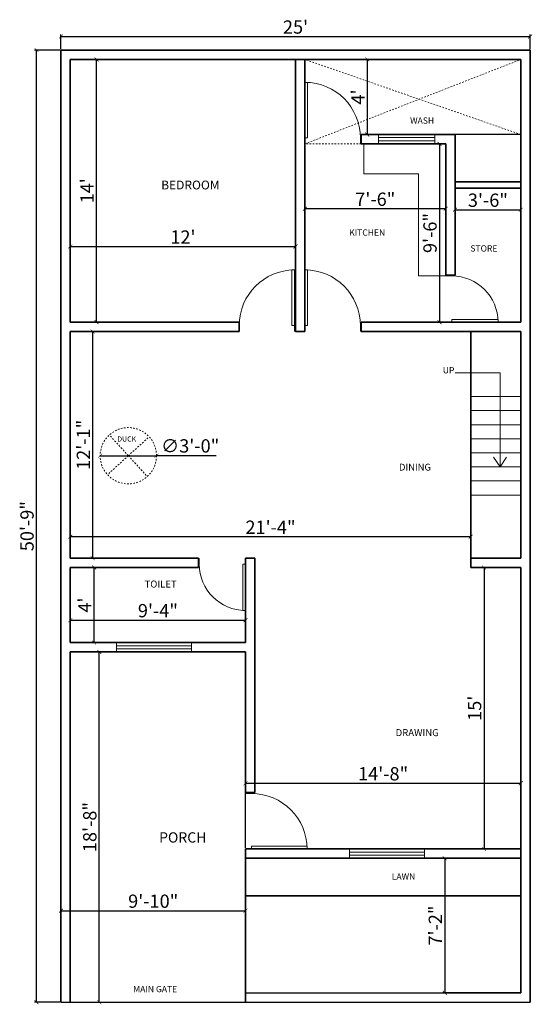
# Model space of a CAD drawing. Units: inches. Extents: x 3799 to 20199, y 1682 to 8087.
# Tile 22 of 30: x 12191 to 12519, y 6979 to 7609. Entities that reach past the tile are written whole.
import ezdxf

# ---------------------------------------------------------------- set-up
doc = ezdxf.new("R2010")
doc.units = ezdxf.units.IN
doc.linetypes.add('JIS_02_1.0', pattern=[2, 1, -1])
for name, color, linetype, lineweight in [('A-ANNO-DIMS', 2, 'Continuous', 18), ('A-ANNO-SYMB', 3, 'Continuous', 18), ('A-AREA-IDEN', 7, 'Continuous', 18), ('A-DOOR', 3, 'Continuous', 18), ('A-FLOR-CASE', 32, 'Continuous', 18), ('A-FLOR-SHFT-HIDN', 8, 'JIS_02_1.0', 13), ('A-FLOR-STRS', 41, 'Continuous', 18), ('A-GLAZ', 152, 'Continuous', 18), ('A-WALL', 7, 'Continuous', 35), ('A-WALL-OVHD', 7, 'JIS_02_1.0', 18), ('C-PROP', 7, 'Continuous', 25)]:
    doc.layers.add(name, color=color, linetype=linetype, lineweight=lineweight)
doc.styles.get("Standard").update_dxf_attribs({"font": 'arial.ttf'})
doc.dimstyles.new('ISO-25', dxfattribs={"dimtxt": 8.5, "dimasz": 2.5, "dimexe": 1.25, "dimexo": 0.625, "dimtad": 1, "dimdec": 0, "dimlunit": 3, "dimtxsty": 'Standard', "dimblk": 'ARCHTICK', "dimcen": 2.5, "dimadec": 0, "dimazin": 0, "dimtfac": 1, "dimtdec": 0, "dimtmove": 0, "dimatfit": 3, "dimfxl": 1, "dimarcsym": 0})

# ---------------------------------------------------------------- blocks, each defined once
blk = doc.blocks.new('_ArchTick')
at = {"color": 0, "linetype": 'ByBlock', "const_width": 0.15}
blk.add_lwpolyline([(-0.5, -0.5), (0.5, 0.5)], dxfattribs=at)
blk = doc.blocks.new('*D177')
at = {"layer": 'A-ANNO-DIMS', "color": 0, "lineweight": -2, "transparency": 16777216}
for p, q in [((12217.15, 7590.06), (12217.15, 7599.38)), ((12217.15, 7598.13), (12517.15, 7598.13)), ((12517.15, 7590.06), (12517.15, 7599.38))]:
    blk.add_line(p, q, dxfattribs=at)
at = {"layer": 'Defpoints', "color": 0, "transparency": 16777216}
for p in [(12517.15, 7598.13), (12217.15, 7589.44), (12517.15, 7589.44)]:
    blk.add_point(p, dxfattribs=at)
at = {"layer": 'A-ANNO-DIMS', "color": 0, "lineweight": -2, "transparency": 16777216, "xscale": 2.5, "yscale": 2.5, "zscale": 2.5, "rotation": 180}
blk.add_blockref('_ArchTick', (12217.15, 7598.13), dxfattribs=at)
at = {"layer": 'A-ANNO-DIMS', "color": 0, "lineweight": -2, "transparency": 16777216, "xscale": 2.5, "yscale": 2.5, "zscale": 2.5}
blk.add_blockref('_ArchTick', (12517.15, 7598.13), dxfattribs=at)
at = {"layer": 'A-ANNO-DIMS', "color": 0, "transparency": 16777216, "insert": (12367.15, 7603.1), "char_height": 8.5, "attachment_point": 5}
blk.add_mtext("25'", dxfattribs=at)
blk = doc.blocks.new('*D178')
at = {"layer": 'A-ANNO-DIMS', "color": 0, "lineweight": -2, "transparency": 16777216}
for p, q in [((12216.53, 7589.44), (12200.29, 7589.44)), ((12201.54, 6980.44), (12201.54, 7589.44)), ((12216.53, 6980.44), (12200.29, 6980.44))]:
    blk.add_line(p, q, dxfattribs=at)
at = {"layer": 'Defpoints', "color": 0, "transparency": 16777216}
for p in [(12201.54, 7589.44), (12217.15, 7589.44), (12217.15, 6980.44)]:
    blk.add_point(p, dxfattribs=at)
at = {"layer": 'A-ANNO-DIMS', "color": 0, "lineweight": -2, "transparency": 16777216, "xscale": 2.5, "yscale": 2.5, "zscale": 2.5}
for p, rotation in [((12201.54, 7589.44), 90), ((12201.54, 6980.44), 270)]:
    blk.add_blockref('_ArchTick', p, dxfattribs=dict(at, rotation=rotation))
at = {"layer": 'A-ANNO-DIMS', "color": 0, "transparency": 16777216, "insert": (12196.57, 7284.94), "char_height": 8.5, "attachment_point": 5, "rotation": 90}
blk.add_mtext('50\'-9"', dxfattribs=at)
blk = doc.blocks.new('*U49')
for p, q in [((0, 0), (0, -100)), ((900, 0), (900, -100))]:
    blk.add_line(p, q)
blk.add_lwpolyline([(0, 0), (0, 900), (43.75, 900), (43.75, 0)], close=True)
blk.add_arc((0, 0), 900, 0, 90)
blk = doc.blocks.new('*U171')
for p, q in [((-750, 0), (-750, 100)), ((0, 0), (0, 100))]:
    blk.add_line(p, q)
blk.add_lwpolyline([(0, 0), (0, -750), (-43.75, -750), (-43.75, 0)], close=True)
blk.add_arc((0, 0), 750, 180, 270)
blk = doc.blocks.new('*U179')
for p, q in [((0, 0), (0, -100)), ((-900, 0), (-900, -100))]:
    blk.add_line(p, q)
blk.add_lwpolyline([(0, 0), (0, 900), (-43.75, 900), (-43.75, 0)], close=True)
blk.add_arc((0, 0), 900, 90, 180)
blk = doc.blocks.new('*U148')
for p, q in [((-750, 0), (-750, -100)), ((0, 0), (0, -100))]:
    blk.add_line(p, q)
blk.add_lwpolyline([(0, 0), (0, 750), (-43.75, 750), (-43.75, 0)], close=True)
blk.add_arc((0, 0), 750, 90, 180)
blk = doc.blocks.new('*D181')
at = {"layer": 'A-ANNO-DIMS', "color": 0, "lineweight": -2, "transparency": 16777216}
for p, q in [((12223.78, 7583.44), (12241.14, 7583.44)), ((12239.89, 7415.44), (12239.89, 7583.44)), ((12223.78, 7415.44), (12241.14, 7415.44))]:
    blk.add_line(p, q, dxfattribs=at)
at = {"layer": 'Defpoints', "color": 0, "transparency": 16777216}
for p in [(12223.15, 7583.44), (12239.89, 7583.44), (12223.15, 7415.44)]:
    blk.add_point(p, dxfattribs=at)
at = {"layer": 'A-ANNO-DIMS', "color": 0, "lineweight": -2, "transparency": 16777216, "xscale": 2.5, "yscale": 2.5, "zscale": 2.5}
for p, rotation in [((12239.89, 7583.44), 90), ((12239.89, 7415.44), 270)]:
    blk.add_blockref('_ArchTick', p, dxfattribs=dict(at, rotation=rotation))
at = {"layer": 'A-ANNO-DIMS', "color": 0, "transparency": 16777216, "insert": (12235, 7499.44), "char_height": 8.5, "attachment_point": 5, "rotation": 90}
blk.add_mtext("14'", dxfattribs=at)
blk = doc.blocks.new('*D182')
at = {"layer": 'A-ANNO-DIMS', "color": 0, "lineweight": -2, "transparency": 16777216}
for p, q in [((12223.15, 7582.81), (12223.15, 7462.61)), ((12367.15, 7582.81), (12367.15, 7462.61)), ((12223.15, 7463.86), (12367.15, 7463.86))]:
    blk.add_line(p, q, dxfattribs=at)
at = {"layer": 'Defpoints', "color": 0, "transparency": 16777216}
for p in [(12223.15, 7583.44), (12367.15, 7583.44), (12367.15, 7463.86)]:
    blk.add_point(p, dxfattribs=at)
at = {"layer": 'A-ANNO-DIMS', "color": 0, "lineweight": -2, "transparency": 16777216, "xscale": 2.5, "yscale": 2.5, "zscale": 2.5, "rotation": 180}
blk.add_blockref('_ArchTick', (12223.15, 7463.86), dxfattribs=at)
at = {"layer": 'A-ANNO-DIMS', "color": 0, "lineweight": -2, "transparency": 16777216, "xscale": 2.5, "yscale": 2.5, "zscale": 2.5}
blk.add_blockref('_ArchTick', (12367.15, 7463.86), dxfattribs=at)
at = {"layer": 'A-ANNO-DIMS', "color": 0, "transparency": 16777216, "insert": (12295.15, 7468.75), "char_height": 8.5, "attachment_point": 5}
blk.add_mtext("12'", dxfattribs=at)
blk = doc.blocks.new('*D183')
at = {"layer": 'A-ANNO-DIMS', "color": 0, "lineweight": -2, "transparency": 16777216}
for p, q in [((12510.53, 7583.44), (12411.75, 7583.44)), ((12413, 7583.44), (12413, 7535.44)), ((12510.53, 7535.44), (12411.75, 7535.44))]:
    blk.add_line(p, q, dxfattribs=at)
at = {"layer": 'Defpoints', "color": 0, "transparency": 16777216}
for p in [(12511.15, 7583.44), (12413, 7535.44), (12511.15, 7535.44)]:
    blk.add_point(p, dxfattribs=at)
at = {"layer": 'A-ANNO-DIMS', "color": 0, "lineweight": -2, "transparency": 16777216, "xscale": 2.5, "yscale": 2.5, "zscale": 2.5}
for p, rotation in [((12413, 7583.44), 90), ((12413, 7535.44), 270)]:
    blk.add_blockref('_ArchTick', p, dxfattribs=dict(at, rotation=rotation))
at = {"layer": 'A-ANNO-DIMS', "color": 0, "transparency": 16777216, "insert": (12408.12, 7559.44), "char_height": 8.5, "attachment_point": 5, "rotation": 90}
blk.add_mtext("4'", dxfattribs=at)
blk = doc.blocks.new('*D184')
at = {"layer": 'A-ANNO-DIMS', "color": 0, "lineweight": -2, "transparency": 16777216}
for p, q in [((12373.15, 7446.06), (12373.15, 7489.23)), ((12463.15, 7446.06), (12463.15, 7489.23)), ((12463.15, 7487.98), (12373.15, 7487.98))]:
    blk.add_line(p, q, dxfattribs=at)
at = {"layer": 'Defpoints', "color": 0, "transparency": 16777216}
for p in [(12373.15, 7487.98), (12373.15, 7445.44), (12463.15, 7445.44)]:
    blk.add_point(p, dxfattribs=at)
at = {"layer": 'A-ANNO-DIMS', "color": 0, "lineweight": -2, "transparency": 16777216, "xscale": 2.5, "yscale": 2.5, "zscale": 2.5, "rotation": 180}
blk.add_blockref('_ArchTick', (12373.15, 7487.98), dxfattribs=at)
at = {"layer": 'A-ANNO-DIMS', "color": 0, "lineweight": -2, "transparency": 16777216, "xscale": 2.5, "yscale": 2.5, "zscale": 2.5}
blk.add_blockref('_ArchTick', (12463.15, 7487.98), dxfattribs=at)
at = {"layer": 'A-ANNO-DIMS', "color": 0, "transparency": 16777216, "insert": (12418.15, 7492.95), "char_height": 8.5, "attachment_point": 5}
blk.add_mtext('7\'-6"', dxfattribs=at)
blk = doc.blocks.new('*D185')
at = {"layer": 'A-ANNO-DIMS', "color": 0, "lineweight": -2, "transparency": 16777216}
for p, q in [((12462.53, 7529.44), (12457.95, 7529.44)), ((12459.2, 7529.44), (12459.2, 7415.44)), ((12462.53, 7415.44), (12457.95, 7415.44))]:
    blk.add_line(p, q, dxfattribs=at)
at = {"layer": 'Defpoints', "color": 0, "transparency": 16777216}
for p in [(12463.15, 7529.44), (12459.2, 7415.44), (12463.15, 7415.44)]:
    blk.add_point(p, dxfattribs=at)
at = {"layer": 'A-ANNO-DIMS', "color": 0, "lineweight": -2, "transparency": 16777216, "xscale": 2.5, "yscale": 2.5, "zscale": 2.5}
for p, rotation in [((12459.2, 7529.44), 90), ((12459.2, 7415.44), 270)]:
    blk.add_blockref('_ArchTick', p, dxfattribs=dict(at, rotation=rotation))
at = {"layer": 'A-ANNO-DIMS', "color": 0, "transparency": 16777216, "insert": (12454.24, 7472.44), "char_height": 8.5, "attachment_point": 5, "rotation": 90}
blk.add_mtext('9\'-6"', dxfattribs=at)
blk = doc.blocks.new('*D186')
at = {"layer": 'A-ANNO-DIMS', "color": 0, "lineweight": -2, "transparency": 16777216}
for p, q in [((12469.15, 7500.59), (12469.15, 7486.11)), ((12511.15, 7500.59), (12511.15, 7486.11)), ((12469.15, 7487.36), (12511.15, 7487.36))]:
    blk.add_line(p, q, dxfattribs=at)
at = {"layer": 'Defpoints', "color": 0, "transparency": 16777216}
for p in [(12469.15, 7501.21), (12511.15, 7501.21), (12511.15, 7487.36)]:
    blk.add_point(p, dxfattribs=at)
at = {"layer": 'A-ANNO-DIMS', "color": 0, "lineweight": -2, "transparency": 16777216, "xscale": 2.5, "yscale": 2.5, "zscale": 2.5, "rotation": 180}
blk.add_blockref('_ArchTick', (12469.15, 7487.36), dxfattribs=at)
at = {"layer": 'A-ANNO-DIMS', "color": 0, "lineweight": -2, "transparency": 16777216, "xscale": 2.5, "yscale": 2.5, "zscale": 2.5}
blk.add_blockref('_ArchTick', (12511.15, 7487.36), dxfattribs=at)
at = {"layer": 'A-ANNO-DIMS', "color": 0, "transparency": 16777216, "insert": (12490.15, 7492.33), "char_height": 8.5, "attachment_point": 5}
blk.add_mtext('3\'-6"', dxfattribs=at)
blk = doc.blocks.new('*D187')
at = {"layer": 'A-ANNO-DIMS', "color": 0, "lineweight": -2, "transparency": 16777216}
for p, q in [((12223.78, 7409.44), (12238.72, 7409.44)), ((12237.47, 7264.44), (12237.47, 7409.44)), ((12223.78, 7264.44), (12238.72, 7264.44))]:
    blk.add_line(p, q, dxfattribs=at)
at = {"layer": 'Defpoints', "color": 0, "transparency": 16777216}
for p in [(12223.15, 7409.44), (12237.47, 7409.44), (12223.15, 7264.44)]:
    blk.add_point(p, dxfattribs=at)
at = {"layer": 'A-ANNO-DIMS', "color": 0, "lineweight": -2, "transparency": 16777216, "xscale": 2.5, "yscale": 2.5, "zscale": 2.5}
for p, rotation in [((12237.47, 7409.44), 90), ((12237.47, 7264.44), 270)]:
    blk.add_blockref('_ArchTick', p, dxfattribs=dict(at, rotation=rotation))
at = {"layer": 'A-ANNO-DIMS', "color": 0, "transparency": 16777216, "insert": (12232.58, 7336.94), "char_height": 8.5, "attachment_point": 5, "rotation": 90}
blk.add_mtext('12\'-1"', dxfattribs=at)
blk = doc.blocks.new('*D188')
at = {"layer": 'A-ANNO-DIMS', "color": 0, "lineweight": -2, "transparency": 16777216}
for p, q in [((12223.15, 7265.06), (12223.15, 7279.48)), ((12223.15, 7278.23), (12479.15, 7278.23)), ((12479.15, 7265.06), (12479.15, 7279.48))]:
    blk.add_line(p, q, dxfattribs=at)
at = {"layer": 'Defpoints', "color": 0, "transparency": 16777216}
for p in [(12479.15, 7278.23), (12223.15, 7264.44), (12479.15, 7264.44)]:
    blk.add_point(p, dxfattribs=at)
at = {"layer": 'A-ANNO-DIMS', "color": 0, "lineweight": -2, "transparency": 16777216, "xscale": 2.5, "yscale": 2.5, "zscale": 2.5, "rotation": 180}
blk.add_blockref('_ArchTick', (12223.15, 7278.23), dxfattribs=at)
at = {"layer": 'A-ANNO-DIMS', "color": 0, "lineweight": -2, "transparency": 16777216, "xscale": 2.5, "yscale": 2.5, "zscale": 2.5}
blk.add_blockref('_ArchTick', (12479.15, 7278.23), dxfattribs=at)
at = {"layer": 'A-ANNO-DIMS', "color": 0, "transparency": 16777216, "insert": (12351.15, 7283.12), "char_height": 8.5, "attachment_point": 5}
blk.add_mtext('21\'-4"', dxfattribs=at)
blk = doc.blocks.new('*D189')
at = {"layer": 'A-ANNO-DIMS', "color": 0, "lineweight": -2, "transparency": 16777216}
for p, q in [((12223.78, 7258.44), (12239.64, 7258.44)), ((12238.39, 7210.44), (12238.39, 7258.44)), ((12223.78, 7210.44), (12239.64, 7210.44))]:
    blk.add_line(p, q, dxfattribs=at)
at = {"layer": 'Defpoints', "color": 0, "transparency": 16777216}
for p in [(12223.15, 7258.44), (12238.39, 7258.44), (12223.15, 7210.44)]:
    blk.add_point(p, dxfattribs=at)
at = {"layer": 'A-ANNO-DIMS', "color": 0, "lineweight": -2, "transparency": 16777216, "xscale": 2.5, "yscale": 2.5, "zscale": 2.5}
for p, rotation in [((12238.39, 7258.44), 90), ((12238.39, 7210.44), 270)]:
    blk.add_blockref('_ArchTick', p, dxfattribs=dict(at, rotation=rotation))
at = {"layer": 'A-ANNO-DIMS', "color": 0, "transparency": 16777216, "insert": (12233.52, 7234.44), "char_height": 8.5, "attachment_point": 5, "rotation": 90}
blk.add_mtext("4'", dxfattribs=at)
blk = doc.blocks.new('*D190')
at = {"layer": 'A-ANNO-DIMS', "color": 0, "lineweight": -2, "transparency": 16777216}
for p, q in [((12223.15, 7211.06), (12223.15, 7226.05)), ((12223.15, 7224.8), (12335.15, 7224.8)), ((12335.15, 7211.06), (12335.15, 7226.05))]:
    blk.add_line(p, q, dxfattribs=at)
at = {"layer": 'Defpoints', "color": 0, "transparency": 16777216}
for p in [(12335.15, 7224.8), (12223.15, 7210.44), (12335.15, 7210.44)]:
    blk.add_point(p, dxfattribs=at)
at = {"layer": 'A-ANNO-DIMS', "color": 0, "lineweight": -2, "transparency": 16777216, "xscale": 2.5, "yscale": 2.5, "zscale": 2.5, "rotation": 180}
blk.add_blockref('_ArchTick', (12223.15, 7224.8), dxfattribs=at)
at = {"layer": 'A-ANNO-DIMS', "color": 0, "lineweight": -2, "transparency": 16777216, "xscale": 2.5, "yscale": 2.5, "zscale": 2.5}
blk.add_blockref('_ArchTick', (12335.15, 7224.8), dxfattribs=at)
at = {"layer": 'A-ANNO-DIMS', "color": 0, "transparency": 16777216, "insert": (12279.15, 7229.76), "char_height": 8.5, "attachment_point": 5}
blk.add_mtext('9\'-4"', dxfattribs=at)
blk = doc.blocks.new('*D191')
at = {"layer": 'A-ANNO-DIMS', "color": 0, "lineweight": -2, "transparency": 16777216}
for p, q in [((12223.78, 7204.44), (12242.92, 7204.44)), ((12241.67, 6980.44), (12241.67, 7204.44)), ((12223.78, 6980.44), (12242.92, 6980.44))]:
    blk.add_line(p, q, dxfattribs=at)
at = {"layer": 'Defpoints', "color": 0, "transparency": 16777216}
for p in [(12223.15, 7204.44), (12241.67, 7204.44), (12223.15, 6980.44)]:
    blk.add_point(p, dxfattribs=at)
at = {"layer": 'A-ANNO-DIMS', "color": 0, "lineweight": -2, "transparency": 16777216, "xscale": 2.5, "yscale": 2.5, "zscale": 2.5}
for p, rotation in [((12241.67, 7204.44), 90), ((12241.67, 6980.44), 270)]:
    blk.add_blockref('_ArchTick', p, dxfattribs=dict(at, rotation=rotation))
at = {"layer": 'A-ANNO-DIMS', "color": 0, "transparency": 16777216, "insert": (12236.71, 7092.44), "char_height": 8.5, "attachment_point": 5, "rotation": 90}
blk.add_mtext('18\'-8"', dxfattribs=at)
blk = doc.blocks.new('*D192')
at = {"layer": 'A-ANNO-DIMS', "color": 0, "lineweight": -2, "transparency": 16777216}
for p, q in [((12217.15, 6981.06), (12217.15, 7040.2)), ((12217.15, 7038.95), (12335.15, 7038.95)), ((12335.15, 6981.06), (12335.15, 7040.2))]:
    blk.add_line(p, q, dxfattribs=at)
at = {"layer": 'Defpoints', "color": 0, "transparency": 16777216}
for p in [(12335.15, 7038.95), (12217.15, 6980.44), (12335.15, 6980.44)]:
    blk.add_point(p, dxfattribs=at)
at = {"layer": 'A-ANNO-DIMS', "color": 0, "lineweight": -2, "transparency": 16777216, "xscale": 2.5, "yscale": 2.5, "zscale": 2.5, "rotation": 180}
blk.add_blockref('_ArchTick', (12217.15, 7038.95), dxfattribs=at)
at = {"layer": 'A-ANNO-DIMS', "color": 0, "lineweight": -2, "transparency": 16777216, "xscale": 2.5, "yscale": 2.5, "zscale": 2.5}
blk.add_blockref('_ArchTick', (12335.15, 7038.95), dxfattribs=at)
at = {"layer": 'A-ANNO-DIMS', "color": 0, "transparency": 16777216, "insert": (12276.15, 7043.92), "char_height": 8.5, "attachment_point": 5}
blk.add_mtext('9\'-10"', dxfattribs=at)
blk = doc.blocks.new('*D193')
at = {"layer": 'A-ANNO-DIMS', "color": 0, "lineweight": -2, "transparency": 16777216}
for p, q in [((12510.53, 7072.44), (12461.27, 7072.44)), ((12462.52, 7072.44), (12462.52, 6986.44)), ((12510.53, 6986.44), (12461.27, 6986.44))]:
    blk.add_line(p, q, dxfattribs=at)
at = {"layer": 'Defpoints', "color": 0, "transparency": 16777216}
for p in [(12511.15, 7072.44), (12462.52, 6986.44), (12511.15, 6986.44)]:
    blk.add_point(p, dxfattribs=at)
at = {"layer": 'A-ANNO-DIMS', "color": 0, "lineweight": -2, "transparency": 16777216, "xscale": 2.5, "yscale": 2.5, "zscale": 2.5}
for p, rotation in [((12462.52, 7072.44), 90), ((12462.52, 6986.44), 270)]:
    blk.add_blockref('_ArchTick', p, dxfattribs=dict(at, rotation=rotation))
at = {"layer": 'A-ANNO-DIMS', "color": 0, "transparency": 16777216, "insert": (12457.63, 7029.44), "char_height": 8.5, "attachment_point": 5, "rotation": 90}
blk.add_mtext('7\'-2"', dxfattribs=at)
blk = doc.blocks.new('*D194')
at = {"layer": 'A-ANNO-DIMS', "color": 0, "lineweight": -2, "transparency": 16777216}
for p, q in [((12510.53, 7258.44), (12486.45, 7258.44)), ((12487.7, 7258.44), (12487.7, 7078.44)), ((12510.53, 7078.44), (12486.45, 7078.44))]:
    blk.add_line(p, q, dxfattribs=at)
at = {"layer": 'Defpoints', "color": 0, "transparency": 16777216}
for p in [(12511.15, 7258.44), (12487.7, 7078.44), (12511.15, 7078.44)]:
    blk.add_point(p, dxfattribs=at)
at = {"layer": 'A-ANNO-DIMS', "color": 0, "lineweight": -2, "transparency": 16777216, "xscale": 2.5, "yscale": 2.5, "zscale": 2.5}
for p, rotation in [((12487.7, 7258.44), 90), ((12487.7, 7078.44), 270)]:
    blk.add_blockref('_ArchTick', p, dxfattribs=dict(at, rotation=rotation))
at = {"layer": 'A-ANNO-DIMS', "color": 0, "transparency": 16777216, "insert": (12482.74, 7168.44), "char_height": 8.5, "attachment_point": 5, "rotation": 90}
blk.add_mtext("15'", dxfattribs=at)
blk = doc.blocks.new('*D195')
at = {"layer": 'A-ANNO-DIMS', "color": 0, "lineweight": -2, "transparency": 16777216}
for p, q in [((12335.15, 7079.06), (12335.15, 7121.68)), ((12335.15, 7120.43), (12511.15, 7120.43)), ((12511.15, 7079.06), (12511.15, 7121.68))]:
    blk.add_line(p, q, dxfattribs=at)
at = {"layer": 'Defpoints', "color": 0, "transparency": 16777216}
for p in [(12511.15, 7120.43), (12335.15, 7078.44), (12511.15, 7078.44)]:
    blk.add_point(p, dxfattribs=at)
at = {"layer": 'A-ANNO-DIMS', "color": 0, "lineweight": -2, "transparency": 16777216, "xscale": 2.5, "yscale": 2.5, "zscale": 2.5, "rotation": 180}
blk.add_blockref('_ArchTick', (12335.15, 7120.43), dxfattribs=at)
at = {"layer": 'A-ANNO-DIMS', "color": 0, "lineweight": -2, "transparency": 16777216, "xscale": 2.5, "yscale": 2.5, "zscale": 2.5}
blk.add_blockref('_ArchTick', (12511.15, 7120.43), dxfattribs=at)
at = {"layer": 'A-ANNO-DIMS', "color": 0, "transparency": 16777216, "insert": (12423.15, 7125.4), "char_height": 8.5, "attachment_point": 5}
blk.add_mtext('14\'-8"', dxfattribs=at)
blk = doc.blocks.new('WIN-48IN-6IN-FRAME')
for p, q in [((0, 0), (0, 6)), ((48, 4), (0, 4)), ((48, 2), (0, 2)), ((48, 0), (48, 6))]:
    blk.add_line(p, q)
blk = doc.blocks.new('WIN-36IN-6IN-FRAME')
for p, q in [((0, 0), (0, 6)), ((36, 4), (0, 4)), ((36, 2), (0, 2)), ((36, 0), (36, 6))]:
    blk.add_line(p, q)
blk = doc.blocks.new('*D390')
at = {"layer": 'A-ANNO-DIMS', "color": 0, "lineweight": -2, "transparency": 16777216}
for p in [(12242.24, 7329.97), (12316.33, 7329.97)]:
    blk.add_line(p, (12278.24, 7329.97), dxfattribs=at)
at = {"layer": 'Defpoints', "color": 0, "transparency": 16777216}
for p in [(12242.24, 7329.97), (12278.24, 7329.97)]:
    blk.add_point(p, dxfattribs=at)
at = {"layer": 'A-ANNO-DIMS', "color": 0, "lineweight": -2, "transparency": 16777216, "xscale": 2.5, "yscale": 2.5, "zscale": 2.5}
for p, rotation in [((12242.24, 7329.97), 359.9985930703019), ((12278.24, 7329.97), 179.9985930703018)]:
    blk.add_blockref('_ArchTick', p, dxfattribs=dict(at, rotation=rotation))
at = {"layer": 'A-ANNO-DIMS', "color": 0, "transparency": 16777216, "insert": (12299.78, 7335.17), "char_height": 8.5, "attachment_point": 5, "rotation": 359.99859}
blk.add_mtext('∅3\'-0"', dxfattribs=at)

msp = doc.modelspace()

# ---------------------------------------------------------------- linework, layer by layer
at = {"layer": 'A-FLOR-CASE'}
for p, q in [((12410.74, 7510.24), (12410.74, 7529.44)), ((12445.84, 7510.24), (12410.74, 7510.24)), ((12445.84, 7444.97), (12445.84, 7510.24)), ((12463.15, 7444.97), (12445.84, 7444.97))]:
    msp.add_line(p, q, dxfattribs=at)
at = {"layer": 'A-FLOR-SHFT-HIDN'}
for q in [(12248.11, 7343.28), (12273.54, 7342.09), (12246.93, 7317.85), (12272.36, 7316.66)]:
    msp.add_line((12260.24, 7329.97), q, dxfattribs=at)
msp.add_circle((12260.24, 7329.97), 18, dxfattribs=at)
at = {"layer": 'A-FLOR-STRS'}
for p, q in [((12469.3, 7382.93), (12497.92, 7382.93)), ((12497.92, 7382.93), (12497.92, 7322.82)), ((12511.15, 7367.82), (12479.15, 7367.82)), ((12511.15, 7358.82), (12479.15, 7358.82)), ((12511.15, 7349.82), (12479.15, 7349.82)), ((12511.15, 7340.82), (12479.15, 7340.82)), ((12511.15, 7331.82), (12479.15, 7331.82)), ((12497.92, 7322.82), (12493.75, 7329.09)), ((12497.92, 7322.82), (12502.08, 7329.09)), ((12511.15, 7322.82), (12479.15, 7322.82)), ((12511.15, 7313.82), (12479.15, 7313.82)), ((12511.15, 7304.82), (12479.15, 7304.82))]:
    msp.add_line(p, q, dxfattribs=at)
at = {"layer": 'A-WALL'}
for p, q in [((12217.15, 7589.44), (12517.15, 7589.44)), ((12217.15, 6980.44), (12217.15, 7589.44)), ((12223.15, 7583.44), (12373.15, 7583.44)), ((12223.15, 7415.44), (12223.15, 7583.44)), ((12367.15, 7409.44), (12367.15, 7583.44)), ((12373.15, 7409.44), (12373.15, 7583.44)), ((12373.15, 7583.44), (12511.15, 7583.44)), ((12511.15, 7583.44), (12511.15, 7415.44)), ((12517.15, 7589.44), (12517.15, 6980.44)), ((12409.15, 7535.44), (12469.15, 7535.44)), ((12409.15, 7529.44), (12409.15, 7535.44)), ((12469.15, 7535.44), (12469.15, 7445.44)), ((12409.15, 7529.44), (12463.15, 7529.44)), ((12463.15, 7529.44), (12463.15, 7445.44)), ((12469.15, 7505.21), (12511.15, 7505.21)), ((12469.15, 7501.21), (12511.15, 7501.21)), ((12463.15, 7445.44), (12469.15, 7445.44)), ((12223.15, 7415.44), (12331.15, 7415.44)), ((12331.15, 7409.44), (12331.15, 7415.44)), ((12409.15, 7415.44), (12511.15, 7415.44)), ((12409.15, 7409.44), (12409.15, 7415.44)), ((12223.15, 7409.44), (12331.15, 7409.44)), ((12223.15, 7264.44), (12223.15, 7409.44)), ((12367.15, 7409.44), (12373.15, 7409.44)), ((12409.15, 7409.44), (12511.15, 7409.44)), ((12479.15, 7258.44), (12479.15, 7409.44)), ((12511.15, 7409.44), (12511.15, 7264.44)), ((12223.15, 7264.44), (12305.15, 7264.44)), ((12305.15, 7258.44), (12305.15, 7264.44)), ((12335.15, 7258.44), (12335.15, 7264.44)), ((12335.15, 7264.44), (12341.15, 7264.44)), ((12341.15, 7114.44), (12341.15, 7264.44)), ((12479.15, 7264.44), (12511.15, 7264.44)), ((12223.15, 7258.44), (12305.15, 7258.44)), ((12223.15, 7210.44), (12223.15, 7258.44)), ((12335.15, 7210.44), (12335.15, 7258.44)), ((12479.15, 7258.44), (12511.15, 7258.44)), ((12511.15, 7258.44), (12511.15, 6986.44)), ((12223.15, 7210.44), (12335.15, 7210.44)), ((12223.15, 6980.44), (12223.15, 7204.44)), ((12223.15, 7204.44), (12335.15, 7204.44)), ((12335.15, 7114.44), (12335.15, 7204.44)), ((12335.15, 7114.44), (12341.15, 7114.44)), ((12335.15, 6980.44), (12335.15, 7078.44)), ((12335.15, 7078.44), (12511.15, 7078.44)), ((12335.15, 7072.44), (12511.15, 7072.44)), ((12335.15, 7048.44), (12511.15, 7048.44))]:
    msp.add_line(p, q, dxfattribs=at)
at = {"layer": 'A-WALL-OVHD'}
for p, q in [((12511.15, 7535.44), (12373.15, 7583.44)), ((12373.15, 7529.44), (12511.15, 7583.44)), ((12469.15, 7535.44), (12511.15, 7535.44)), ((12409.15, 7529.44), (12373.15, 7529.44))]:
    msp.add_line(p, q, dxfattribs=at)
at = {"layer": 'C-PROP'}
for p, q in [((12335.15, 6986.44), (12511.15, 6986.44)), ((12217.15, 6980.44), (12335.15, 6980.44)), ((12335.15, 6980.44), (12517.15, 6980.44))]:
    msp.add_line(p, q, dxfattribs=at)

# ---------------------------------------------------------------- block references
at = {"layer": 'A-DOOR', "xscale": 0.0393700787401575, "yscale": 0.0393700787401575, "zscale": 0.0393700787401575}
for name, p in [('*U49', (12373.15, 7533.38)), ('*U179', (12366.59, 7413.38)), ('*U49', (12373.15, 7413.38)), ('*U171', (12335.15, 7260.5))]:
    msp.add_blockref(name, p, dxfattribs=at)
at = {"layer": 'A-DOOR', "xscale": 0.0393700787401575, "yscale": 0.0393700787401575, "zscale": 0.0393700787401575, "rotation": 270}
for name, p in [('*U148', (12467.09, 7415.44)), ('*U179', (12339.09, 7078.44))]:
    msp.add_blockref(name, p, dxfattribs=at)
at = {"layer": 'A-GLAZ'}
for name, p in [('WIN-36IN-6IN-FRAME', (12420.17, 7529.44)), ('WIN-48IN-6IN-FRAME', (12252.73, 7204.44)), ('WIN-48IN-6IN-FRAME', (12401.61, 7072.44))]:
    msp.add_blockref(name, p, dxfattribs=at)

# ---------------------------------------------------------------- texts
at = {"layer": 'A-ANNO-SYMB'}
msp.add_text('UP', height=4, rotation=0.00083, dxfattribs=at).set_placement((12461.31, 7382.63))
at = {"layer": 'A-AREA-IDEN'}
for s, height, p in [('WASH', 4, (12440.41, 7542.36)), ('BEDROOM', 5.626, (12281.25, 7500.33)), ('KITCHEN', 4, (12401.44, 7470.73)), ('STORE', 4, (12478.95, 7460.58)), ('DUCK', 3.278, (12253.16, 7339.04)), ('DINING', 4.381, (12433.32, 7320.47)), ('TOILET', 4.49, (12270.59, 7245.63)), ('DRAWING', 4.478, (12431.16, 7150.59)), ('PORCH', 6.564, (12279.91, 7082.52)), ('LAWN', 4, (12428.69, 7058.81)), ('MAIN GATE', 4, (12263.38, 6986.8))]:
    msp.add_text(s, height=height, rotation=0.00083, dxfattribs=at).set_placement(p)

# ---------------------------------------------------------------- dimensions: what is measured, and where the dimension line sits
at = {"layer": 'A-ANNO-DIMS'}
for base, p1, p2, picture, middle in [((12517.15, 7598.13), (12217.15, 7589.44), (12517.15, 7589.44), '*D177', (12367.15, 7603.1)), ((12367.15, 7463.86), (12223.15, 7583.44), (12367.15, 7583.44), '*D182', (12295.15, 7468.75)), ((12373.15, 7487.98), (12463.15, 7445.44), (12373.15, 7445.44), '*D184', (12418.15, 7492.95)), ((12511.15, 7487.36), (12469.15, 7501.21), (12511.15, 7501.21), '*D186', (12490.15, 7492.33)), ((12479.15, 7278.23), (12223.15, 7264.44), (12479.15, 7264.44), '*D188', (12351.15, 7283.12)), ((12335.15, 7224.8), (12223.15, 7210.44), (12335.15, 7210.44), '*D190', (12279.15, 7229.76)), ((12511.15, 7120.43), (12335.15, 7078.44), (12511.15, 7078.44), '*D195', (12423.15, 7125.4)), ((12335.15, 7038.95), (12217.15, 6980.44), (12335.15, 6980.44), '*D192', (12276.15, 7043.92))]:
    dim = msp.add_linear_dim(base=base, p1=p1, p2=p2, dimstyle='ISO-25', override={"dimclrd": 0, "dimclre": 0, "dimclrt": 0}, dxfattribs=at)
    dim.commit()
    dim.dimension.update_dxf_attribs({"geometry": picture, "text_midpoint": middle})
for base, p1, p2, picture, middle in [((12201.54, 7589.44), (12217.15, 6980.44), (12217.15, 7589.44), '*D178', (12196.57, 7284.94)), ((12239.89, 7583.44), (12223.15, 7415.44), (12223.15, 7583.44), '*D181', (12235, 7499.44)), ((12413, 7535.44), (12511.15, 7583.44), (12511.15, 7535.44), '*D183', (12408.12, 7559.44)), ((12459.2, 7415.44), (12463.15, 7529.44), (12463.15, 7415.44), '*D185', (12454.24, 7472.44)), ((12237.47, 7409.44), (12223.15, 7264.44), (12223.15, 7409.44), '*D187', (12232.58, 7336.94)), ((12238.39, 7258.44), (12223.15, 7210.44), (12223.15, 7258.44), '*D189', (12233.52, 7234.44)), ((12487.7, 7078.44), (12511.15, 7258.44), (12511.15, 7078.44), '*D194', (12482.74, 7168.44)), ((12241.67, 7204.44), (12223.15, 6980.44), (12223.15, 7204.44), '*D191', (12236.71, 7092.44)), ((12462.52, 6986.44), (12511.15, 7072.44), (12511.15, 6986.44), '*D193', (12457.63, 7029.44))]:
    dim = msp.add_linear_dim(base=base, p1=p1, p2=p2, angle=90, dimstyle='ISO-25', override={"dimclrd": 0, "dimclre": 0, "dimclrt": 0}, dxfattribs=at)
    dim.commit()
    dim.dimension.update_dxf_attribs({"geometry": picture, "text_midpoint": middle})
dim = msp.add_diameter_dim_2p(p1=(12242.24, 7329.97), p2=(12278.24, 7329.97), dimstyle='ISO-25', override={"dimdec": 1, "dimlfac": 1, "dimrnd": 0, "dimzin": 1, "dimdsep": 46, "dimlunit": 4, "dimfrac": 2}, dxfattribs=at)
dim.commit()
dim.dimension.update_dxf_attribs({"geometry": '*D390', "text_midpoint": (12299.78, 7329.97), "dimtype": 163})

doc.saveas('drawing.dxf')
